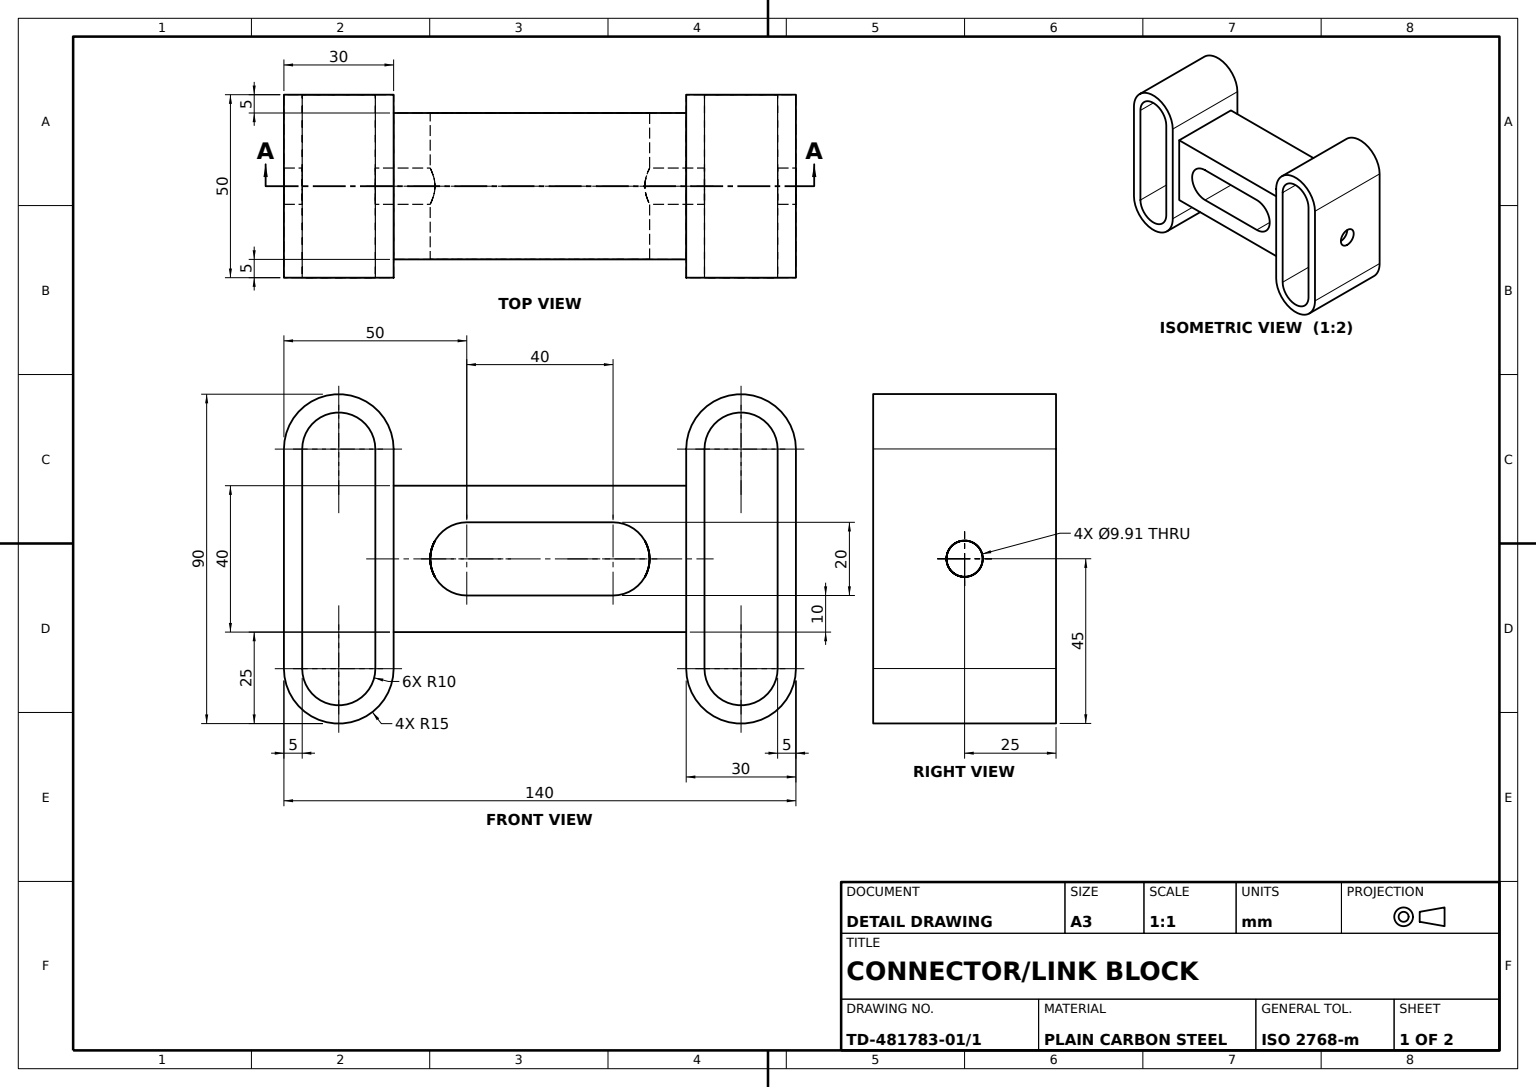
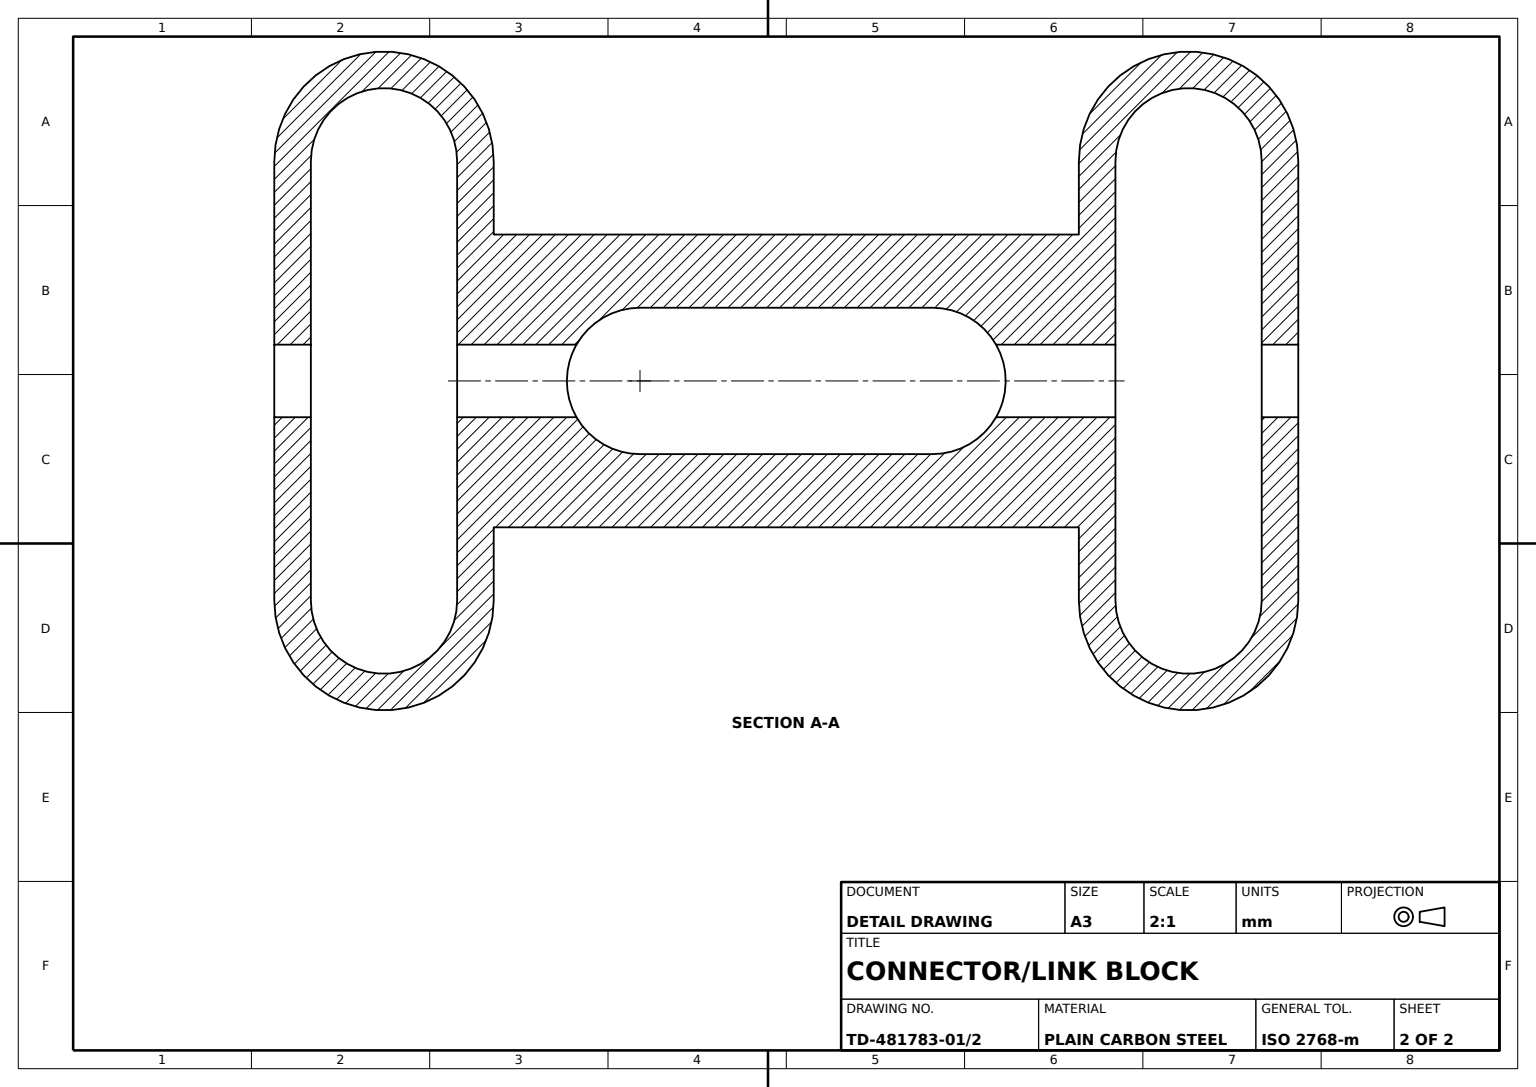
from build123d import *

# Parameters (mm, degrees)
END_LOOPS_DEPTH       = 25
END_LOOPS_2_DEPTH     = 25
CENTRE_BLOCK_SKETCH_W = 80
CENTRE_BLOCK_SKETCH_H = 40
CENTRE_BLOCK_DEPTH    = 20
CROSS_HOLE_SKETCH_R   = 4.957337167
CROSS_HOLE_DEPTH      = 164


with BuildPart() as part:
    # End Loops Sketch → End Loops (new, symmetric)
    with BuildSketch(Plane.XY):
        with BuildLine():
            Line((-40, 35), (-40, -25))
            ThreePointArc((-40, -25), (-55, -40), (-70, -25))
            Line((-70, -25), (-70, 35))
            ThreePointArc((-70, 35), (-55, 50), (-40, 35))
        make_face()
        with BuildLine():
            Line((-45, 35), (-45, -25))
            ThreePointArc((-45, -25), (-55, -35), (-65, -25))
            Line((-65, -25), (-65, 35))
            ThreePointArc((-65, 35), (-55, 45), (-45, 35))
        make_face(mode=Mode.SUBTRACT)
    extrude(amount=END_LOOPS_DEPTH, both=True)



with BuildPart() as body_2:
    # End Loops Sketch → End Loops 2 (new, symmetric)
    with BuildSketch(Plane.XY):
        with BuildLine():
            Line((70, 35), (70, -25))
            ThreePointArc((70, -25), (55, -40), (40, -25))
            Line((40, -25), (40, 35))
            ThreePointArc((40, 35), (55, 50), (70, 35))
        make_face()
        with BuildLine():
            Line((65, 35), (65, -25))
            ThreePointArc((65, -25), (55, -35), (45, -25))
            Line((45, -25), (45, 35))
            ThreePointArc((45, 35), (55, 45), (65, 35))
        make_face(mode=Mode.SUBTRACT)
    extrude(amount=END_LOOPS_2_DEPTH, both=True)


with BuildPart() as part_1:
    add(part.part)

    add(body_2.part)  # Centre Block merges body 2
    # Centre Block Sketch → Centre Block (add, symmetric)
    with BuildSketch(Plane.XY):
        with Locations((0, 5)):
            Rectangle(CENTRE_BLOCK_SKETCH_W, CENTRE_BLOCK_SKETCH_H)
        with BuildLine():
            Line((-20, 15), (20, 15))
            ThreePointArc((20, 15), (30, 5), (20, -5))
            Line((20, -5), (-20, -5))
            ThreePointArc((-20, -5), (-30, 5), (-20, 15))
        make_face(mode=Mode.SUBTRACT)
    extrude(amount=CENTRE_BLOCK_DEPTH, both=True)

    # Cross Hole Sketch → Cross Hole (cut)
    with BuildSketch(Plane(origin=(70, 0, 0), x_dir=(0, 0, -1), z_dir=(1, 0, 0))):
        with Locations(Location((0, 5, 0), (0, 0, 90))):
            Circle(CROSS_HOLE_SKETCH_R)
    extrude(amount=-CROSS_HOLE_DEPTH, mode=Mode.SUBTRACT)


solid = part_1.part
